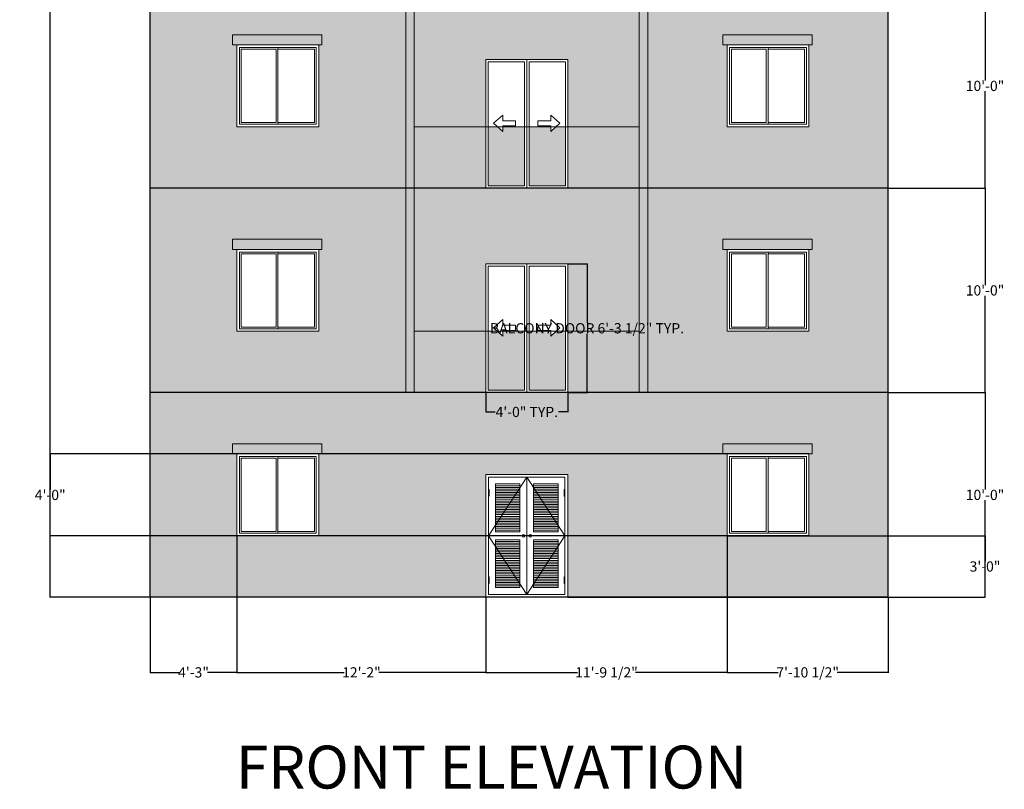
# Model space of a CAD drawing. Units: inches. Extents: x -113 to 5399, y -1393 to 3302.
# Tile 20 of 40: x 3613 to 4191, y -1393 to -941. Entities that reach past the tile are written whole.
import ezdxf

# ---------------------------------------------------------------- set-up
doc = ezdxf.new("R2010")
doc.units = ezdxf.units.IN
doc.header["$MEASUREMENT"] = 0
for name, color, linetype, lineweight in [('A-ANNO-DIMS', 254, 'Continuous', 18), ('A-ANNO-TEXT', 7, 'Continuous', 25), ('A-Door', 150, 'Continuous', 18), ('A-ELEV', 7, 'Continuous', 25), ('A-ELEV-GLAZ', 150, 'Continuous', 18), ('A-ELEV-RAIL', 7, 'Continuous', 18), ('A-ELEV-TRIM', 7, 'Continuous', 18), ('A-ELEV-TRIM-PATT', 7, 'Continuous', 13)]:
    doc.layers.add(name, color=color, linetype=linetype, lineweight=lineweight)
doc.layers.add('A-ELEV-RAIL-PATT', color=9, linetype='Continuous', lineweight=13, true_color=0xc7c8ca)
doc.layers.add('A-ELEV-WALL-PATT', color=241, linetype='Continuous', lineweight=13, true_color=0xf7abae)
doc.styles.get("Standard").update_dxf_attribs({"font": 'arial.ttf'})
doc.dimstyles.get("Standard").update_dxf_attribs({"dimtxt": 6, "dimasz": 0.18, "dimexe": 0.18, "dimexo": 0.0625, "dimgap": 0.09, "dimtad": 0, "dimtih": 1, "dimtoh": 1, "dimdec": 1, "dimzin": 0, "dimdsep": 46, "dimlunit": 4, "dimtxsty": 'Standard', "dimblk": 'ARCHTICK', "dimcen": 0.09, "dimadec": 0, "dimazin": 0, "dimtfac": 1, "dimtdec": 1, "dimtofl": 0, "dimtmove": 0, "dimatfit": 3, "dimfxl": 1, "dimtolj": 1, "dimtzin": 0, "dimarcsym": 0})

# ---------------------------------------------------------------- blocks, each defined once
blk = doc.blocks.new('AE0C11')
for p, q in [((0, 0), (0, 1800)), ((0, 1800), (1200, 1800)), ((40, 40), (40, 1760)), ((40, 1760), (1160, 1760)), ((600, 1760), (40, 900)), ((600, 40), (600, 1760)), ((600, 1760), (1160, 900)), ((1160, 40), (1160, 1760)), ((1200, 0), (1200, 1800)), ((140, 1660), (500, 1660)), ((140, 960), (140, 1660)), ((140, 1635), (500, 1635)), ((140, 1610), (500, 1610)), ((500, 960), (500, 1660)), ((700, 960), (700, 1660)), ((1060, 1660), (700, 1660)), ((1060, 1635), (700, 1635)), ((1060, 1610), (700, 1610)), ((1060, 960), (1060, 1660)), ((40, 1580), (50, 1580)), ((40, 1480), (50, 1480)), ((50, 1480), (50, 1580)), ((140, 1585), (500, 1585)), ((140, 1560), (500, 1560)), ((140, 1535), (500, 1535)), ((140, 1510), (500, 1510)), ((140, 1485), (500, 1485)), ((140, 1460), (500, 1460)), ((1060, 1585), (700, 1585)), ((1060, 1560), (700, 1560)), ((1060, 1535), (700, 1535)), ((1060, 1510), (700, 1510)), ((1060, 1485), (700, 1485)), ((1060, 1460), (700, 1460)), ((1150, 1480), (1150, 1580)), ((1150, 1580), (1160, 1580)), ((1150, 1480), (1160, 1480)), ((140, 1435), (500, 1435)), ((140, 1410), (500, 1410)), ((140, 1385), (500, 1385)), ((140, 1360), (500, 1360)), ((140, 1335), (500, 1335)), ((140, 1310), (500, 1310)), ((1060, 1435), (700, 1435)), ((1060, 1410), (700, 1410)), ((1060, 1385), (700, 1385)), ((1060, 1360), (700, 1360)), ((1060, 1335), (700, 1335)), ((1060, 1310), (700, 1310)), ((140, 1285), (500, 1285)), ((140, 1260), (500, 1260)), ((140, 1235), (500, 1235)), ((140, 1210), (500, 1210)), ((140, 1185), (500, 1185)), ((140, 1160), (500, 1160)), ((1060, 1285), (700, 1285)), ((1060, 1260), (700, 1260)), ((1060, 1235), (700, 1235)), ((1060, 1210), (700, 1210)), ((1060, 1185), (700, 1185)), ((1060, 1160), (700, 1160)), ((140, 1135), (500, 1135)), ((140, 1110), (500, 1110)), ((140, 1085), (500, 1085)), ((140, 1060), (500, 1060)), ((140, 1035), (500, 1035)), ((1060, 1135), (700, 1135)), ((1060, 1110), (700, 1110)), ((1060, 1085), (700, 1085)), ((1060, 1060), (700, 1060)), ((1060, 1035), (700, 1035)), ((40, 900), (600, 40)), ((140, 1010), (500, 1010)), ((140, 985), (500, 985)), ((140, 960), (500, 960)), ((1160, 900), (600, 40)), ((1060, 1010), (700, 1010)), ((1060, 985), (700, 985)), ((1060, 960), (700, 960)), ((140, 840), (500, 840)), ((140, 840), (140, 140)), ((140, 815), (500, 815)), ((140, 790), (500, 790)), ((140, 765), (500, 765)), ((140, 740), (500, 740)), ((500, 840), (500, 140)), ((700, 840), (700, 140)), ((1060, 840), (700, 840)), ((1060, 815), (700, 815)), ((1060, 790), (700, 790)), ((1060, 765), (700, 765)), ((1060, 740), (700, 740)), ((1060, 840), (1060, 140)), ((140, 715), (500, 715)), ((140, 690), (500, 690)), ((140, 665), (500, 665)), ((140, 640), (500, 640)), ((140, 615), (500, 615)), ((140, 590), (500, 590)), ((1060, 715), (700, 715)), ((1060, 690), (700, 690)), ((1060, 665), (700, 665)), ((1060, 640), (700, 640)), ((1060, 615), (700, 615)), ((1060, 590), (700, 590)), ((140, 565), (500, 565)), ((140, 540), (500, 540)), ((140, 515), (500, 515)), ((140, 490), (500, 490)), ((140, 465), (500, 465)), ((140, 440), (500, 440)), ((1060, 565), (700, 565)), ((1060, 540), (700, 540)), ((1060, 515), (700, 515)), ((1060, 490), (700, 490)), ((1060, 465), (700, 465)), ((1060, 440), (700, 440)), ((50, 300), (40, 300)), ((50, 200), (50, 300)), ((140, 415), (500, 415)), ((140, 390), (500, 390)), ((140, 365), (500, 365)), ((140, 340), (500, 340)), ((140, 315), (500, 315)), ((140, 290), (500, 290)), ((1060, 415), (700, 415)), ((1060, 390), (700, 390)), ((1060, 365), (700, 365)), ((1060, 340), (700, 340)), ((1060, 315), (700, 315)), ((1060, 290), (700, 290)), ((1150, 300), (1160, 300)), ((1150, 200), (1150, 300)), ((50, 200), (40, 200)), ((140, 265), (500, 265)), ((140, 240), (500, 240)), ((140, 215), (500, 215)), ((140, 190), (500, 190)), ((140, 165), (500, 165)), ((1060, 265), (700, 265)), ((1060, 240), (700, 240)), ((1060, 215), (700, 215)), ((1060, 190), (700, 190)), ((1060, 165), (700, 165)), ((1150, 200), (1160, 200)), ((0, 0), (1200, 0)), ((40, 40), (1160, 40)), ((140, 140), (500, 140)), ((1060, 140), (700, 140))]:
    blk.add_line(p, q)
for centre in [(550, 900), (650, 900)]:
    blk.add_circle(centre, 20)
blk = doc.blocks.new('*U84')
for p, q in [((1.5, 1.5), (1.5, 46.5)), ((1.5, 46.5), (24, 46.5)), ((24, 1.5), (24, 46.5)), ((24, 46.5), (46.5, 46.5)), ((46.5, 46.5), (46.5, 1.5)), ((24, 1.5), (1.5, 1.5)), ((46.5, 1.5), (24, 1.5))]:
    blk.add_line(p, q)
blk.add_lwpolyline([(0, 0), (0, 48), (48, 48), (48, 0)], close=True)
for points in [[(23, 45.5), (23, 2.5), (2.5, 2.5), (2.5, 45.5), (23, 45.5)], [(24, 45.5), (45.5, 45.5), (45.5, 2.5), (24, 2.5)]]:
    blk.add_lwpolyline(points)
blk = doc.blocks.new('DOOR-SLIDING-PAIR-ELEV')
for p, q in [((9.94, 42.86), (4.53, 38.04)), ((9.94, 39.54), (9.94, 42.86)), ((38.06, 39.54), (38.06, 42.86)), ((38.06, 42.86), (43.47, 38.04)), ((9.94, 33.21), (4.53, 38.04)), ((17.43, 39.54), (9.94, 39.54)), ((17.43, 36.54), (9.94, 36.54)), ((9.94, 36.54), (9.94, 33.21)), ((17.43, 39.54), (17.43, 36.54)), ((30.57, 39.54), (38.06, 39.54)), ((30.57, 39.54), (30.57, 36.54)), ((30.57, 36.54), (38.06, 36.54)), ((38.06, 33.21), (43.47, 38.04)), ((38.06, 36.54), (38.06, 33.21))]:
    blk.add_line(p, q)
for points in [[(0, 75.57), (24, 75.57), (24, 0), (0, 0)], [(24, 75.57), (48, 75.57), (48, 0), (24, 0)], [(1.37, 74.2), (22.63, 74.2), (22.63, 1.37), (1.37, 1.37)], [(25.37, 74.2), (46.63, 74.2), (46.63, 1.37), (25.37, 1.37)]]:
    blk.add_lwpolyline(points, close=True)
blk = doc.blocks.new('_ArchTick')
at = {"color": 0, "linetype": 'ByBlock', "const_width": 0.15}
blk.add_lwpolyline([(-0.5, -0.5), (0.5, 0.5)], dxfattribs=at)
blk = doc.blocks.new('*D189')
at = {"layer": 'A-ANNO-DIMS', "color": 0, "lineweight": -2, "transparency": 16777216}
for p, q in [((3934.79, -1084.56), (3946.25, -1084.56)), ((3946.07, -1084.56), (3946.07, -1119.15)), ((3946.07, -1160.13), (3946.07, -1125.54)), ((3934.79, -1160.13), (3946.25, -1160.13))]:
    blk.add_line(p, q, dxfattribs=at)
at = {"layer": 'Defpoints', "color": 0, "transparency": 16777216}
for p in [(3934.73, -1084.56), (3946.07, -1084.56), (3934.73, -1160.13)]:
    blk.add_point(p, dxfattribs=at)
at = {"layer": 'A-ANNO-DIMS', "color": 0, "lineweight": -2, "transparency": 16777216, "xscale": 0.18, "yscale": 0.18, "zscale": 0.18}
for p, rotation in [((3946.07, -1084.56), 90), ((3946.07, -1160.13), 270)]:
    blk.add_blockref('_ArchTick', p, dxfattribs=dict(at, rotation=rotation))
at = {"layer": 'A-ANNO-DIMS', "color": 0, "transparency": 16777216, "insert": (3946.07, -1122.35), "char_height": 6, "attachment_point": 5}
blk.add_mtext('\\A1;BALCONY DOOR 6\'-3 1/2" TYP.', dxfattribs=at)
blk = doc.blocks.new('*D190')
at = {"layer": 'A-ANNO-DIMS', "color": 0, "lineweight": -2, "transparency": 16777216}
for p, q in [((3886.73, -1160.2), (3886.73, -1171.65)), ((3934.73, -1160.2), (3934.73, -1171.65)), ((3886.73, -1171.47), (3892.23, -1171.47)), ((3934.73, -1171.47), (3929.23, -1171.47))]:
    blk.add_line(p, q, dxfattribs=at)
at = {"layer": 'Defpoints', "color": 0, "transparency": 16777216}
for p in [(3886.73, -1160.13), (3934.73, -1160.13), (3934.73, -1171.47)]:
    blk.add_point(p, dxfattribs=at)
at = {"layer": 'A-ANNO-DIMS', "color": 0, "lineweight": -2, "transparency": 16777216, "xscale": 0.18, "yscale": 0.18, "zscale": 0.18, "rotation": 180}
blk.add_blockref('_ArchTick', (3886.73, -1171.47), dxfattribs=at)
at = {"layer": 'A-ANNO-DIMS', "color": 0, "lineweight": -2, "transparency": 16777216, "xscale": 0.18, "yscale": 0.18, "zscale": 0.18}
blk.add_blockref('_ArchTick', (3934.73, -1171.47), dxfattribs=at)
at = {"layer": 'A-ANNO-DIMS', "color": 0, "transparency": 16777216, "insert": (3910.73, -1171.47), "char_height": 6, "attachment_point": 5}
blk.add_mtext('\\A1;4\'-0" TYP.', dxfattribs=at)
blk = doc.blocks.new('*D214')
at = {"layer": 'A-ANNO-DIMS', "color": 0, "lineweight": -2, "transparency": 16777216}
for p, q in [((3725.67, -555.41), (3631, -555.41)), ((3631.18, -555.41), (3631.18, -914.58)), ((3631.18, -1280.13), (3631.18, -920.96)), ((3689.67, -1280.13), (3631, -1280.13))]:
    blk.add_line(p, q, dxfattribs=at)
at = {"layer": 'Defpoints', "color": 0, "transparency": 16777216}
for p in [(3631.18, -555.41), (3725.73, -555.41), (3689.73, -1280.13)]:
    blk.add_point(p, dxfattribs=at)
at = {"layer": 'A-ANNO-DIMS', "color": 0, "lineweight": -2, "transparency": 16777216, "xscale": 0.18, "yscale": 0.18, "zscale": 0.18}
for p, rotation in [((3631.18, -555.41), 90), ((3631.18, -1280.13), 270)]:
    blk.add_blockref('_ArchTick', p, dxfattribs=dict(at, rotation=rotation))
at = {"layer": 'A-ANNO-DIMS', "color": 0, "transparency": 16777216, "insert": (3631.18, -917.77), "char_height": 6, "attachment_point": 5}
blk.add_mtext('\\A1;60\'-4 1/2"', dxfattribs=at)
blk = doc.blocks.new('*D215')
at = {"layer": 'A-ANNO-DIMS', "color": 0, "lineweight": -2, "transparency": 16777216}
for p, q in [((3740.73, -1244.2), (3740.73, -1324.46)), ((3689.73, -1280.2), (3689.73, -1324.46)), ((3689.73, -1324.28), (3707.04, -1324.28)), ((3740.73, -1324.28), (3723.41, -1324.28))]:
    blk.add_line(p, q, dxfattribs=at)
at = {"layer": 'Defpoints', "color": 0, "transparency": 16777216}
for p in [(3740.73, -1244.13), (3689.73, -1280.13), (3740.73, -1324.28)]:
    blk.add_point(p, dxfattribs=at)
at = {"layer": 'A-ANNO-DIMS', "color": 0, "lineweight": -2, "transparency": 16777216, "xscale": 0.18, "yscale": 0.18, "zscale": 0.18, "rotation": 180}
blk.add_blockref('_ArchTick', (3689.73, -1324.28), dxfattribs=at)
at = {"layer": 'A-ANNO-DIMS', "color": 0, "lineweight": -2, "transparency": 16777216, "xscale": 0.18, "yscale": 0.18, "zscale": 0.18}
blk.add_blockref('_ArchTick', (3740.73, -1324.28), dxfattribs=at)
at = {"layer": 'A-ANNO-DIMS', "color": 0, "transparency": 16777216, "insert": (3715.23, -1324.28), "char_height": 6, "attachment_point": 5}
blk.add_mtext('\\A1;4\'-3"', dxfattribs=at)
blk = doc.blocks.new('*D216')
at = {"layer": 'A-ANNO-DIMS', "color": 0, "lineweight": -2, "transparency": 16777216}
for p, q in [((3740.73, -1244.2), (3740.73, -1324.46)), ((3886.73, -1280.2), (3886.73, -1324.46)), ((3740.73, -1324.28), (3803.62, -1324.28)), ((3886.73, -1324.28), (3823.84, -1324.28))]:
    blk.add_line(p, q, dxfattribs=at)
at = {"layer": 'Defpoints', "color": 0, "transparency": 16777216}
for p in [(3740.73, -1244.13), (3886.73, -1280.13), (3886.73, -1324.28)]:
    blk.add_point(p, dxfattribs=at)
at = {"layer": 'A-ANNO-DIMS', "color": 0, "lineweight": -2, "transparency": 16777216, "xscale": 0.18, "yscale": 0.18, "zscale": 0.18, "rotation": 180}
blk.add_blockref('_ArchTick', (3740.73, -1324.28), dxfattribs=at)
at = {"layer": 'A-ANNO-DIMS', "color": 0, "lineweight": -2, "transparency": 16777216, "xscale": 0.18, "yscale": 0.18, "zscale": 0.18}
blk.add_blockref('_ArchTick', (3886.73, -1324.28), dxfattribs=at)
at = {"layer": 'A-ANNO-DIMS', "color": 0, "transparency": 16777216, "insert": (3813.73, -1324.28), "char_height": 6, "attachment_point": 5}
blk.add_mtext('\\A1;12\'-2"', dxfattribs=at)
blk = doc.blocks.new('*D217')
at = {"layer": 'A-ANNO-DIMS', "color": 0, "lineweight": -2, "transparency": 16777216}
for p, q in [((4028.23, -1244.2), (4028.23, -1324.46)), ((3886.73, -1280.2), (3886.73, -1324.46)), ((3886.73, -1324.28), (3940.38, -1324.28)), ((4028.23, -1324.28), (3974.58, -1324.28))]:
    blk.add_line(p, q, dxfattribs=at)
at = {"layer": 'Defpoints', "color": 0, "transparency": 16777216}
for p in [(4028.23, -1244.13), (3886.73, -1280.13), (4028.23, -1324.28)]:
    blk.add_point(p, dxfattribs=at)
at = {"layer": 'A-ANNO-DIMS', "color": 0, "lineweight": -2, "transparency": 16777216, "xscale": 0.18, "yscale": 0.18, "zscale": 0.18, "rotation": 180}
blk.add_blockref('_ArchTick', (3886.73, -1324.28), dxfattribs=at)
at = {"layer": 'A-ANNO-DIMS', "color": 0, "lineweight": -2, "transparency": 16777216, "xscale": 0.18, "yscale": 0.18, "zscale": 0.18}
blk.add_blockref('_ArchTick', (4028.23, -1324.28), dxfattribs=at)
at = {"layer": 'A-ANNO-DIMS', "color": 0, "transparency": 16777216, "insert": (3957.48, -1324.28), "char_height": 6, "attachment_point": 5}
blk.add_mtext('\\A1;11\'-9 1/2"', dxfattribs=at)
blk = doc.blocks.new('*D218')
at = {"layer": 'A-ANNO-DIMS', "color": 0, "lineweight": -2, "transparency": 16777216}
for p, q in [((4028.23, -1244.2), (4028.23, -1324.46)), ((4122.73, -1280.2), (4122.73, -1324.46)), ((4028.23, -1324.28), (4058.12, -1324.28)), ((4122.73, -1324.28), (4092.84, -1324.28))]:
    blk.add_line(p, q, dxfattribs=at)
at = {"layer": 'Defpoints', "color": 0, "transparency": 16777216}
for p in [(4028.23, -1244.13), (4122.73, -1280.13), (4122.73, -1324.28)]:
    blk.add_point(p, dxfattribs=at)
at = {"layer": 'A-ANNO-DIMS', "color": 0, "lineweight": -2, "transparency": 16777216, "xscale": 0.18, "yscale": 0.18, "zscale": 0.18, "rotation": 180}
blk.add_blockref('_ArchTick', (4028.23, -1324.28), dxfattribs=at)
at = {"layer": 'A-ANNO-DIMS', "color": 0, "lineweight": -2, "transparency": 16777216, "xscale": 0.18, "yscale": 0.18, "zscale": 0.18}
blk.add_blockref('_ArchTick', (4122.73, -1324.28), dxfattribs=at)
at = {"layer": 'A-ANNO-DIMS', "color": 0, "transparency": 16777216, "insert": (4075.48, -1324.28), "char_height": 6, "attachment_point": 5}
blk.add_mtext('\\A1;7\'-10 1/2"', dxfattribs=at)
blk = doc.blocks.new('*D219')
at = {"layer": 'A-ANNO-DIMS', "color": 0, "lineweight": -2, "transparency": 16777216}
for p, q in [((4076.17, -1196.13), (3631, -1196.13)), ((3631.18, -1196.13), (3631.18, -1216.98)), ((3631.18, -1244.13), (3631.18, -1223.29)), ((4076.17, -1244.13), (3631, -1244.13))]:
    blk.add_line(p, q, dxfattribs=at)
at = {"layer": 'Defpoints', "color": 0, "transparency": 16777216}
for p in [(3631.18, -1196.13), (4076.23, -1196.13), (4076.23, -1244.13)]:
    blk.add_point(p, dxfattribs=at)
at = {"layer": 'A-ANNO-DIMS', "color": 0, "lineweight": -2, "transparency": 16777216, "xscale": 0.18, "yscale": 0.18, "zscale": 0.18}
for p, rotation in [((3631.18, -1196.13), 90), ((3631.18, -1244.13), 270)]:
    blk.add_blockref('_ArchTick', p, dxfattribs=dict(at, rotation=rotation))
at = {"layer": 'A-ANNO-DIMS', "color": 0, "transparency": 16777216, "insert": (3631.18, -1220.13), "char_height": 6, "attachment_point": 5}
blk.add_mtext('\\A1;4\'-0"', dxfattribs=at)
blk = doc.blocks.new('*D220')
at = {"layer": 'A-ANNO-DIMS', "color": 0, "lineweight": -2, "transparency": 16777216}
for p, q in [((4028.29, -1244.13), (4179.71, -1244.13)), ((4179.53, -1244.13), (4179.53, -1258.98)), ((4179.53, -1280.13), (4179.53, -1265.29)), ((3934.79, -1280.13), (4179.71, -1280.13))]:
    blk.add_line(p, q, dxfattribs=at)
at = {"layer": 'Defpoints', "color": 0, "transparency": 16777216}
for p in [(4028.23, -1244.13), (4179.53, -1244.13), (3934.73, -1280.13)]:
    blk.add_point(p, dxfattribs=at)
at = {"layer": 'A-ANNO-DIMS', "color": 0, "lineweight": -2, "transparency": 16777216, "xscale": 0.18, "yscale": 0.18, "zscale": 0.18}
for p, rotation in [((4179.53, -1244.13), 90), ((4179.53, -1280.13), 270)]:
    blk.add_blockref('_ArchTick', p, dxfattribs=dict(at, rotation=rotation))
at = {"layer": 'A-ANNO-DIMS', "color": 0, "transparency": 16777216, "insert": (4179.53, -1262.13), "char_height": 6, "attachment_point": 5}
blk.add_mtext('\\A1;3\'-0"', dxfattribs=at)
blk = doc.blocks.new('*D221')
at = {"layer": 'A-ANNO-DIMS', "color": 0, "lineweight": -2, "transparency": 16777216}
for p, q in [((4122.79, -1160.13), (4179.71, -1160.13)), ((4179.53, -1160.13), (4179.53, -1216.98)), ((4179.53, -1280.13), (4179.53, -1223.29)), ((4122.79, -1280.13), (4179.71, -1280.13))]:
    blk.add_line(p, q, dxfattribs=at)
at = {"layer": 'Defpoints', "color": 0, "transparency": 16777216}
for p in [(4122.73, -1160.13), (4179.53, -1160.13), (4122.73, -1280.13)]:
    blk.add_point(p, dxfattribs=at)
at = {"layer": 'A-ANNO-DIMS', "color": 0, "lineweight": -2, "transparency": 16777216, "xscale": 0.18, "yscale": 0.18, "zscale": 0.18}
for p, rotation in [((4179.53, -1160.13), 90), ((4179.53, -1280.13), 270)]:
    blk.add_blockref('_ArchTick', p, dxfattribs=dict(at, rotation=rotation))
at = {"layer": 'A-ANNO-DIMS', "color": 0, "transparency": 16777216, "insert": (4179.53, -1220.13), "char_height": 6, "attachment_point": 5}
blk.add_mtext('\\A1;10\'-0"', dxfattribs=at)
blk = doc.blocks.new('*D222')
at = {"layer": 'A-ANNO-DIMS', "color": 0, "lineweight": -2, "transparency": 16777216}
for p, q in [((4122.79, -1040.13), (4179.71, -1040.13)), ((4179.53, -1040.13), (4179.53, -1096.98)), ((4179.53, -1160.13), (4179.53, -1103.29)), ((4122.79, -1160.13), (4179.71, -1160.13))]:
    blk.add_line(p, q, dxfattribs=at)
at = {"layer": 'Defpoints', "color": 0, "transparency": 16777216}
for p in [(4122.73, -1040.13), (4179.53, -1040.13), (4122.73, -1160.13)]:
    blk.add_point(p, dxfattribs=at)
at = {"layer": 'A-ANNO-DIMS', "color": 0, "lineweight": -2, "transparency": 16777216, "xscale": 0.18, "yscale": 0.18, "zscale": 0.18}
for p, rotation in [((4179.53, -1040.13), 90), ((4179.53, -1160.13), 270)]:
    blk.add_blockref('_ArchTick', p, dxfattribs=dict(at, rotation=rotation))
at = {"layer": 'A-ANNO-DIMS', "color": 0, "transparency": 16777216, "insert": (4179.53, -1100.13), "char_height": 6, "attachment_point": 5}
blk.add_mtext('\\A1;10\'-0"', dxfattribs=at)
blk = doc.blocks.new('*D223')
at = {"layer": 'A-ANNO-DIMS', "color": 0, "lineweight": -2, "transparency": 16777216}
for p, q in [((4122.79, -920.13), (4179.71, -920.13)), ((4179.53, -920.13), (4179.53, -976.98)), ((4179.53, -1040.13), (4179.53, -983.29)), ((4122.79, -1040.13), (4179.71, -1040.13))]:
    blk.add_line(p, q, dxfattribs=at)
at = {"layer": 'Defpoints', "color": 0, "transparency": 16777216}
for p in [(4122.73, -920.13), (4179.53, -920.13), (4122.73, -1040.13)]:
    blk.add_point(p, dxfattribs=at)
at = {"layer": 'A-ANNO-DIMS', "color": 0, "lineweight": -2, "transparency": 16777216, "xscale": 0.18, "yscale": 0.18, "zscale": 0.18}
for p, rotation in [((4179.53, -920.13), 90), ((4179.53, -1040.13), 270)]:
    blk.add_blockref('_ArchTick', p, dxfattribs=dict(at, rotation=rotation))
at = {"layer": 'A-ANNO-DIMS', "color": 0, "transparency": 16777216, "insert": (4179.53, -980.13), "char_height": 6, "attachment_point": 5}
blk.add_mtext('\\A1;10\'-0"', dxfattribs=at)

msp = doc.modelspace()

# ---------------------------------------------------------------- hatches: boundary and pattern name
at = {"layer": 'A-ELEV-RAIL-PATT', "transparency": 33554498}
h = msp.add_hatch(color=256, dxfattribs=at)
h.dxf.hatch_style = 1
h.paths.add_polyline_path([(3886.73, -1004.13), (3844.73, -1004.13), (3844.73, -1040.13), (3886.73, -1040.13)])
h.paths.add_polyline_path([(3976.73, -1004.13), (3934.73, -1004.13), (3934.73, -1040.13), (3976.73, -1040.13)])
h.paths.add_polyline_path([(3933.36, -1004.13), (3927.91, -1004.13), (3924.79, -1006.92), (3924.79, -1004.13), (3912.1, -1004.13), (3912.1, -1038.76), (3933.36, -1038.76)])
h.paths.add_polyline_path([(3909.36, -1004.13), (3896.67, -1004.13), (3896.67, -1006.92), (3893.55, -1004.13), (3888.1, -1004.13), (3888.1, -1038.76), (3909.36, -1038.76)])
h = msp.add_hatch(color=256, dxfattribs=at)
h.dxf.hatch_style = 1
h.paths.add_polyline_path([(3886.73, -1124.13), (3844.73, -1124.13), (3844.73, -1160.13), (3886.73, -1160.13)])
h.paths.add_polyline_path([(3976.73, -1124.13), (3934.73, -1124.13), (3934.73, -1160.13), (3976.73, -1160.13)])
h.paths.add_polyline_path([(3933.36, -1124.13), (3927.91, -1124.13), (3924.79, -1126.92), (3924.79, -1124.13), (3912.1, -1124.13), (3912.1, -1158.76), (3933.36, -1158.76)])
h.paths.add_polyline_path([(3909.36, -1124.13), (3896.67, -1124.13), (3896.67, -1126.92), (3893.55, -1124.13), (3888.1, -1124.13), (3888.1, -1158.76), (3909.36, -1158.76)])
at = {"layer": 'A-ELEV-TRIM-PATT'}
h = msp.add_hatch(color=256, dxfattribs=at)
h.dxf.hatch_style = 1
h.paths.add_polyline_path([(3981.73, -1040.13), (3976.73, -1040.13), (3976.73, -1160.13), (3981.73, -1160.13)])
h.paths.add_polyline_path([(3981.73, -920.13), (3976.73, -920.13), (3976.73, -1040.13), (3981.73, -1040.13)])
h.paths.add_polyline_path([(3981.73, -800.13), (3976.73, -800.13), (3976.73, -920.13), (3981.73, -920.13)])
h.paths.add_polyline_path([(3981.73, -680.13), (3976.73, -680.13), (3976.73, -800.13), (3981.73, -800.13)])
h.paths.add_polyline_path([(3844.73, -680.13), (3839.73, -680.13), (3839.73, -800.13), (3844.73, -800.13)])
h.paths.add_polyline_path([(3844.73, -800.13), (3839.73, -800.13), (3839.73, -920.13), (3844.73, -920.13)])
h.paths.add_polyline_path([(3844.73, -920.13), (3839.73, -920.13), (3839.73, -1040.13), (3844.73, -1040.13)])
h.paths.add_polyline_path([(3844.73, -1040.13), (3839.73, -1040.13), (3839.73, -1160.13), (3844.73, -1160.13)])
h = msp.add_hatch(color=256, dxfattribs=at)
h.dxf.hatch_style = 1
h.paths.add_polyline_path([(4078.05, -1190.14), (4025.64, -1190.14), (4025.64, -1196.13), (4078.05, -1196.13)])
h.paths.add_polyline_path([(3790.55, -1190.14), (3738.14, -1190.14), (3738.14, -1196.13), (3790.55, -1196.13)])
h.paths.add_polyline_path([(3790.55, -1070.14), (3738.14, -1070.14), (3738.14, -1076.13), (3790.55, -1076.13)])
h.paths.add_polyline_path([(3790.55, -950.14), (3738.14, -950.14), (3738.14, -956.13), (3790.55, -956.13)])
h.paths.add_polyline_path([(3790.55, -830.14), (3738.14, -830.14), (3738.14, -836.13), (3790.55, -836.13)])
h.paths.add_polyline_path([(4078.05, -830.14), (4025.64, -830.14), (4025.64, -836.13), (4078.05, -836.13)])
h.paths.add_polyline_path([(4078.05, -710.14), (4025.64, -710.14), (4025.64, -716.13), (4078.05, -716.13)])
h.paths.add_polyline_path([(3790.55, -710.14), (3738.14, -710.14), (3738.14, -716.13), (3790.55, -716.13)])
h.paths.add_polyline_path([(4078.05, -1070.14), (4025.64, -1070.14), (4025.64, -1076.13), (4078.05, -1076.13)])
h.paths.add_polyline_path([(4078.05, -950.14), (4025.64, -950.14), (4025.64, -956.13), (4078.05, -956.13)])
at = {"layer": 'A-ELEV-WALL-PATT'}
h = msp.add_hatch(color=256, dxfattribs=at)
h.dxf.hatch_style = 1
h.paths.add_polyline_path([(3839.73, -680.13), (3689.73, -680.13), (3689.73, -800.13), (3839.73, -800.13)])
h.paths.add_polyline_path([(3790.55, -716.13), (3788.73, -716.13), (3788.73, -764.13), (3740.73, -764.13), (3740.73, -716.13), (3738.14, -716.13), (3738.14, -710.14), (3790.55, -710.14)], flags=16)
h.paths.add_polyline_path([(3787.23, -717.63), (3787.23, -762.63), (3764.73, -762.63), (3742.23, -762.63), (3742.23, -717.63), (3764.73, -717.63)], flags=0)
h.paths.add_polyline_path([(3786.23, -718.63), (3786.23, -761.63), (3764.73, -761.63), (3764.73, -718.63)], flags=0)
h.paths.add_polyline_path([(3763.73, -761.63), (3743.23, -761.63), (3743.23, -718.63), (3763.73, -718.63)], flags=0)
h.paths.add_polyline_path([(3976.73, -680.13), (3844.73, -680.13), (3844.73, -764.13), (3886.73, -764.13), (3886.73, -724.56), (3910.73, -724.56), (3934.73, -724.56), (3934.73, -764.13), (3976.73, -764.13)])
h.paths.add_polyline_path([(4122.73, -680.13), (3981.73, -680.13), (3981.73, -800.13), (4122.73, -800.13)])
h.paths.add_polyline_path([(4028.23, -716.13), (4025.64, -716.13), (4025.64, -710.14), (4078.05, -710.14), (4078.05, -716.13), (4076.23, -716.13), (4076.23, -764.13), (4028.23, -764.13)], flags=16)
h.paths.add_polyline_path([(4029.73, -717.63), (4052.23, -717.63), (4074.73, -717.63), (4074.73, -762.63), (4052.23, -762.63), (4029.73, -762.63)], flags=0)
h.paths.add_polyline_path([(4030.73, -718.63), (4051.23, -718.63), (4051.23, -761.63), (4030.73, -761.63)], flags=0)
h.paths.add_polyline_path([(4052.23, -718.63), (4073.73, -718.63), (4073.73, -761.63), (4052.23, -761.63)], flags=0)
h.paths.add_polyline_path([(4122.73, -800.13), (3981.73, -800.13), (3981.73, -920.13), (4122.73, -920.13)])
h.paths.add_polyline_path([(4025.64, -836.13), (4025.64, -830.14), (4078.05, -830.14), (4078.05, -836.13), (4076.23, -836.13), (4076.23, -884.13), (4028.23, -884.13), (4028.23, -836.13)], flags=16)
h.paths.add_polyline_path([(4029.73, -837.63), (4052.23, -837.63), (4074.73, -837.63), (4074.73, -882.63), (4052.23, -882.63), (4029.73, -882.63)], flags=0)
h.paths.add_polyline_path([(4030.73, -838.63), (4051.23, -838.63), (4051.23, -881.63), (4030.73, -881.63)], flags=0)
h.paths.add_polyline_path([(4052.23, -838.63), (4073.73, -838.63), (4073.73, -881.63), (4052.23, -881.63)], flags=0)
h.paths.add_polyline_path([(3976.73, -800.13), (3844.73, -800.13), (3844.73, -884.13), (3886.73, -884.13), (3886.73, -844.56), (3910.73, -844.56), (3934.73, -844.56), (3934.73, -884.13), (3976.73, -884.13)])
h.paths.add_polyline_path([(3839.73, -800.13), (3689.73, -800.13), (3689.73, -920.13), (3839.73, -920.13)])
h.paths.add_polyline_path([(3788.73, -884.13), (3740.73, -884.13), (3740.73, -836.13), (3738.14, -836.13), (3738.14, -830.14), (3790.55, -830.14), (3790.55, -836.13), (3788.73, -836.13)], flags=16)
h.paths.add_polyline_path([(3787.23, -882.63), (3764.73, -882.63), (3742.23, -882.63), (3742.23, -837.63), (3764.73, -837.63), (3787.23, -837.63)], flags=0)
h.paths.add_polyline_path([(3786.23, -881.63), (3764.73, -881.63), (3764.73, -838.63), (3786.23, -838.63)], flags=0)
h.paths.add_polyline_path([(3763.73, -881.63), (3743.23, -881.63), (3743.23, -838.63), (3763.73, -838.63)], flags=0)
h.paths.add_polyline_path([(3839.73, -920.13), (3689.73, -920.13), (3689.73, -1040.13), (3839.73, -1040.13)])
h.paths.add_polyline_path([(3788.73, -1004.13), (3740.73, -1004.13), (3740.73, -956.13), (3738.14, -956.13), (3738.14, -950.14), (3790.55, -950.14), (3790.55, -956.13), (3788.73, -956.13)], flags=16)
h.paths.add_polyline_path([(3787.23, -1002.63), (3764.73, -1002.63), (3742.23, -1002.63), (3742.23, -957.63), (3764.73, -957.63), (3787.23, -957.63)], flags=0)
h.paths.add_polyline_path([(3786.23, -1001.63), (3764.73, -1001.63), (3764.73, -958.63), (3786.23, -958.63)], flags=0)
h.paths.add_polyline_path([(3763.73, -1001.63), (3743.23, -1001.63), (3743.23, -958.63), (3763.73, -958.63)], flags=0)
h.paths.add_polyline_path([(3976.73, -920.13), (3844.73, -920.13), (3844.73, -1004.13), (3886.73, -1004.13), (3886.73, -964.56), (3910.73, -964.56), (3934.73, -964.56), (3934.73, -1004.13), (3976.73, -1004.13)])
h.paths.add_polyline_path([(4122.73, -920.13), (3981.73, -920.13), (3981.73, -1040.13), (4122.73, -1040.13)])
h.paths.add_polyline_path([(4028.23, -956.13), (4025.64, -956.13), (4025.64, -950.14), (4078.05, -950.14), (4078.05, -956.13), (4076.23, -956.13), (4076.23, -1004.13), (4028.23, -1004.13)], flags=16)
h.paths.add_polyline_path([(4029.73, -957.63), (4052.23, -957.63), (4074.73, -957.63), (4074.73, -1002.63), (4052.23, -1002.63), (4029.73, -1002.63)], flags=0)
h.paths.add_polyline_path([(4030.73, -958.63), (4051.23, -958.63), (4051.23, -1001.63), (4030.73, -1001.63)], flags=0)
h.paths.add_polyline_path([(4052.23, -958.63), (4073.73, -958.63), (4073.73, -1001.63), (4052.23, -1001.63)], flags=0)
h.paths.add_polyline_path([(4122.73, -1040.13), (3981.73, -1040.13), (3981.73, -1160.13), (4122.73, -1160.13)])
h.paths.add_polyline_path([(4028.23, -1076.13), (4025.64, -1076.13), (4025.64, -1070.14), (4078.05, -1070.14), (4078.05, -1076.13), (4076.23, -1076.13), (4076.23, -1124.13), (4028.23, -1124.13)], flags=16)
h.paths.add_polyline_path([(4029.73, -1077.63), (4052.23, -1077.63), (4074.73, -1077.63), (4074.73, -1122.63), (4052.23, -1122.63), (4029.73, -1122.63)], flags=0)
h.paths.add_polyline_path([(4030.73, -1078.63), (4051.23, -1078.63), (4051.23, -1121.63), (4030.73, -1121.63)], flags=0)
h.paths.add_polyline_path([(4052.23, -1078.63), (4073.73, -1078.63), (4073.73, -1121.63), (4052.23, -1121.63)], flags=0)
h.paths.add_polyline_path([(3976.73, -1040.13), (3844.73, -1040.13), (3844.73, -1124.13), (3886.73, -1124.13), (3886.73, -1084.56), (3910.73, -1084.56), (3934.73, -1084.56), (3934.73, -1124.13), (3976.73, -1124.13)])
h.paths.add_polyline_path([(3839.73, -1040.13), (3689.73, -1040.13), (3689.73, -1160.13), (3839.73, -1160.13)])
h.paths.add_polyline_path([(3788.73, -1124.13), (3740.73, -1124.13), (3740.73, -1076.13), (3738.14, -1076.13), (3738.14, -1070.14), (3790.55, -1070.14), (3790.55, -1076.13), (3788.73, -1076.13)], flags=16)
h.paths.add_polyline_path([(3787.23, -1122.63), (3764.73, -1122.63), (3742.23, -1122.63), (3742.23, -1077.63), (3764.73, -1077.63), (3787.23, -1077.63)], flags=0)
h.paths.add_polyline_path([(3786.23, -1121.63), (3764.73, -1121.63), (3764.73, -1078.63), (3786.23, -1078.63)], flags=0)
h.paths.add_polyline_path([(3763.73, -1121.63), (3743.23, -1121.63), (3743.23, -1078.63), (3763.73, -1078.63)], flags=0)
h.paths.add_polyline_path([(3886.73, -1208.13), (3934.73, -1208.13), (3934.73, -1280.13), (4122.73, -1280.13), (4122.73, -1160.13), (3981.73, -1160.13), (3689.73, -1160.13), (3689.73, -1280.13), (3886.73, -1280.13)])
h.paths.add_polyline_path([(3788.73, -1244.13), (3740.73, -1244.13), (3740.73, -1196.13), (3738.14, -1196.13), (3738.14, -1190.14), (3790.55, -1190.14), (3790.55, -1196.13), (3788.73, -1196.13)], flags=16)
h.paths.add_polyline_path([(3787.23, -1242.63), (3764.73, -1242.63), (3742.23, -1242.63), (3742.23, -1197.63), (3764.73, -1197.63), (3787.23, -1197.63)], flags=0)
h.paths.add_polyline_path([(3786.23, -1241.63), (3764.73, -1241.63), (3764.73, -1198.63), (3786.23, -1198.63)], flags=0)
h.paths.add_polyline_path([(3763.73, -1241.63), (3743.23, -1241.63), (3743.23, -1198.63), (3763.73, -1198.63)], flags=0)
h.paths.add_polyline_path([(4025.64, -1196.13), (4025.64, -1190.14), (4078.05, -1190.14), (4078.05, -1196.13), (4076.23, -1196.13), (4076.23, -1244.13), (4028.23, -1244.13), (4028.23, -1196.13)], flags=16)
h.paths.add_polyline_path([(4029.73, -1197.63), (4052.23, -1197.63), (4074.73, -1197.63), (4074.73, -1242.63), (4052.23, -1242.63), (4029.73, -1242.63)], flags=0)
h.paths.add_polyline_path([(4030.73, -1198.63), (4051.23, -1198.63), (4051.23, -1241.63), (4030.73, -1241.63)], flags=0)
h.paths.add_polyline_path([(4052.23, -1198.63), (4073.73, -1198.63), (4073.73, -1241.63), (4052.23, -1241.63)], flags=0)

# ---------------------------------------------------------------- linework, layer by layer
at = {"layer": 'A-Door'}
for p, q in [((3886.73, -1280.13), (3886.73, -1208.13)), ((3934.73, -1280.13), (3934.73, -1208.13))]:
    msp.add_line(p, q, dxfattribs=at)
at = {"layer": 'A-ELEV'}
for p, q in [((3689.73, -1040.13), (3689.73, -920.13)), ((4122.73, -1040.13), (4122.73, -920.13)), ((4122.73, -1040.13), (4122.73, -920.13)), ((3689.73, -1160.13), (3689.73, -1040.13)), ((4122.73, -1040.13), (3689.73, -1040.13)), ((4122.73, -1160.13), (4122.73, -1040.13)), ((4122.73, -1160.13), (4122.73, -1040.13)), ((3689.73, -1280.13), (3689.73, -1160.13)), ((4122.73, -1160.13), (3689.73, -1160.13)), ((4122.73, -1160.13), (3689.73, -1160.13)), ((4122.73, -1160.13), (3689.73, -1160.13)), ((4122.73, -1280.13), (4122.73, -1160.13)), ((4122.73, -1280.13), (3689.73, -1280.13)), ((4122.73, -1280.13), (3689.73, -1280.13))]:
    msp.add_line(p, q, dxfattribs=at)
at = {"layer": 'A-ELEV-GLAZ'}
for p, q in [((3740.73, -1004.13), (3740.73, -956.13)), ((3788.73, -1004.13), (3788.73, -956.13)), ((4028.23, -1004.13), (4028.23, -956.13)), ((4076.23, -1004.13), (4076.23, -956.13)), ((3740.73, -1124.13), (3740.73, -1076.13)), ((3788.73, -1124.13), (3788.73, -1076.13)), ((4028.23, -1124.13), (4028.23, -1076.13)), ((4076.23, -1124.13), (4076.23, -1076.13)), ((3788.73, -1124.13), (3740.73, -1124.13)), ((4076.23, -1124.13), (4028.23, -1124.13)), ((3740.73, -1244.13), (3740.73, -1196.13)), ((3788.73, -1244.13), (3788.73, -1196.13)), ((4028.23, -1244.13), (4028.23, -1196.13)), ((4076.23, -1244.13), (4076.23, -1196.13)), ((3788.73, -1244.13), (3740.73, -1244.13)), ((4076.23, -1244.13), (4028.23, -1244.13))]:
    msp.add_line(p, q, dxfattribs=at)
at = {"layer": 'A-ELEV-RAIL'}
for p, q in [((3844.73, -1004.13), (3976.73, -1004.13)), ((3844.73, -1124.13), (3976.73, -1124.13))]:
    msp.add_line(p, q, dxfattribs=at)
at = {"layer": 'A-ELEV-TRIM'}
for p, q in [((3839.73, -1040.13), (3839.73, -920.13)), ((3844.73, -1040.13), (3844.73, -920.13)), ((3976.73, -1040.13), (3976.73, -920.13)), ((3981.73, -1040.13), (3981.73, -920.13)), ((3839.73, -1160.13), (3839.73, -1040.13)), ((3844.73, -1160.13), (3844.73, -1040.13)), ((3976.73, -1160.13), (3976.73, -1040.13)), ((3981.73, -1160.13), (3981.73, -1040.13))]:
    msp.add_line(p, q, dxfattribs=at)
for points in [[(3738.14, -956.13), (3790.55, -956.13), (3790.55, -950.14), (3738.14, -950.14)], [(4025.64, -956.13), (4078.05, -956.13), (4078.05, -950.14), (4025.64, -950.14)], [(3738.14, -1076.13), (3790.55, -1076.13), (3790.55, -1070.14), (3738.14, -1070.14)], [(4025.64, -1076.13), (4078.05, -1076.13), (4078.05, -1070.14), (4025.64, -1070.14)], [(3738.14, -1196.13), (3790.55, -1196.13), (3790.55, -1190.14), (3738.14, -1190.14)], [(4025.64, -1196.13), (4078.05, -1196.13), (4078.05, -1190.14), (4025.64, -1190.14)]]:
    msp.add_lwpolyline(points, close=True, dxfattribs=at)

# ---------------------------------------------------------------- block references
at = {"layer": 'A-Door'}
for p in [(3886.73, -1040.13), (3886.73, -1160.13)]:
    msp.add_blockref('DOOR-SLIDING-PAIR-ELEV', p, dxfattribs=at)
at = {"layer": 'A-Door', "xscale": 0.0400000000000061, "yscale": 0.0400000000000061, "zscale": 0.0400000000000061}
msp.add_blockref('AE0C11', (3886.73, -1280.13), dxfattribs=at)
at = {"layer": 'A-ELEV-GLAZ'}
for p in [(3740.73, -1004.13), (4028.23, -1004.13), (3740.73, -1124.13), (4028.23, -1124.13), (3740.73, -1244.13), (4028.23, -1244.13)]:
    msp.add_blockref('*U84', p, dxfattribs=at)

# ---------------------------------------------------------------- texts
at = {"layer": 'A-ANNO-TEXT'}
msp.add_text('FRONT ELEVATION', height=25.17, dxfattribs=at).set_placement((3740.09, -1392.44))

# ---------------------------------------------------------------- dimensions: what is measured, and where the dimension line sits
at = {"layer": 'A-ANNO-DIMS'}
for base, p1, p2, picture, middle in [((3631.18, -555.41), (3689.73, -1280.13), (3725.73, -555.41), '*D214', (3631.18, -917.77)), ((4179.53, -920.13), (4122.73, -1040.13), (4122.73, -920.13), '*D223', (4179.53, -980.13)), ((4179.53, -1040.13), (4122.73, -1160.13), (4122.73, -1040.13), '*D222', (4179.53, -1100.13)), ((4179.53, -1160.13), (4122.73, -1280.13), (4122.73, -1160.13), '*D221', (4179.53, -1220.13)), ((3631.18, -1196.13), (4076.23, -1244.13), (4076.23, -1196.13), '*D219', (3631.18, -1220.13)), ((4179.53, -1244.13), (3934.73, -1280.13), (4028.23, -1244.13), '*D220', (4179.53, -1262.13))]:
    dim = msp.add_linear_dim(base=base, p1=p1, p2=p2, angle=90, dimstyle='Standard', override={"dimdec": 1, "dimlfac": 1, "dimrnd": 0, "dimzin": 1, "dimdsep": 46, "dimlunit": 4, "dimfrac": 2}, dxfattribs=at)
    dim.commit()
    dim.dimension.update_dxf_attribs({"geometry": picture, "text_midpoint": middle})
dim = msp.add_linear_dim(base=(3946.07, -1084.56), p1=(3934.73, -1160.13), p2=(3934.73, -1084.56), angle=90, text='BALCONY DOOR <> TYP.', dimstyle='Standard', override={"dimdec": 1, "dimlfac": 1, "dimrnd": 0, "dimzin": 1, "dimdsep": 46, "dimlunit": 4, "dimfrac": 2}, dxfattribs=at)
dim.commit()
dim.dimension.update_dxf_attribs({"geometry": '*D189', "text_midpoint": (3946.07, -1122.35)})
dim = msp.add_linear_dim(base=(3934.73, -1171.47), p1=(3886.73, -1160.13), p2=(3934.73, -1160.13), text='<> TYP.', dimstyle='Standard', override={"dimdec": 1, "dimlfac": 1, "dimrnd": 0, "dimzin": 1, "dimdsep": 46, "dimlunit": 4, "dimfrac": 2}, dxfattribs=at)
dim.commit()
dim.dimension.update_dxf_attribs({"geometry": '*D190', "text_midpoint": (3910.73, -1171.47)})
for base, p1, p2, picture, middle in [((3740.73, -1324.28), (3689.73, -1280.13), (3740.73, -1244.13), '*D215', (3715.23, -1324.28)), ((3886.73, -1324.28), (3740.73, -1244.13), (3886.73, -1280.13), '*D216', (3813.73, -1324.28)), ((4028.23, -1324.28), (3886.73, -1280.13), (4028.23, -1244.13), '*D217', (3957.48, -1324.28)), ((4122.73, -1324.28), (4028.23, -1244.13), (4122.73, -1280.13), '*D218', (4075.48, -1324.28))]:
    dim = msp.add_linear_dim(base=base, p1=p1, p2=p2, dimstyle='Standard', override={"dimdec": 1, "dimlfac": 1, "dimrnd": 0, "dimzin": 1, "dimdsep": 46, "dimlunit": 4, "dimfrac": 2}, dxfattribs=at)
    dim.commit()
    dim.dimension.update_dxf_attribs({"geometry": picture, "text_midpoint": middle})

doc.saveas('drawing.dxf')
